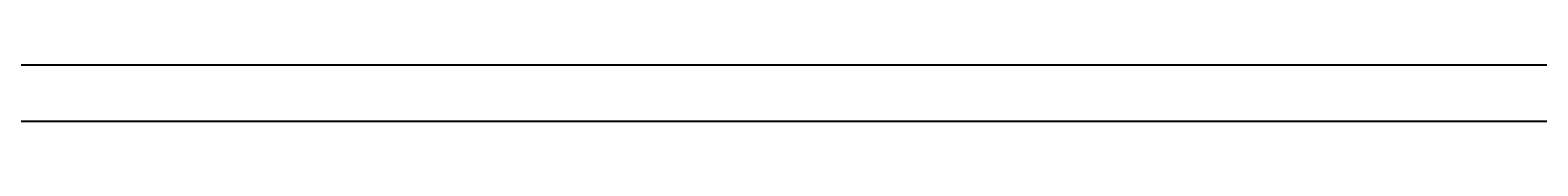
# Model space of a CAD drawing. Units: inches. Extents: x 35362 to 73946, y 43607 to 67532.
# Tile 117 of 134: x 50761 to 50905, y 49313 to 49321. Entities that reach past the tile are written whole.
import ezdxf

# ---------------------------------------------------------------- set-up
doc = ezdxf.new("R2010")
doc.units = ezdxf.units.IN
doc.header["$MEASUREMENT"] = 0
doc.layers.add('A-ANNO-DIMS', color=2, linetype='Continuous', lineweight=18)
doc.styles.get("Standard").update_dxf_attribs({"font": 'arial.ttf'})
doc.dimstyles.get("Standard").update_dxf_attribs({"dimtxt": 0.18, "dimasz": 0.18, "dimexe": 0.18, "dimexo": 0.0625, "dimgap": 0.09, "dimtad": 0, "dimtih": 1, "dimtoh": 1, "dimdec": 4, "dimzin": 0, "dimdsep": 46, "dimtxsty": 'Standard', "dimcen": 0.09, "dimadec": 0, "dimazin": 0, "dimtfac": 1, "dimtdec": 4, "dimtofl": 0, "dimtmove": 0, "dimatfit": 3, "dimfxl": 1, "dimtolj": 1, "dimtzin": 0, "dimarcsym": 0})

# ---------------------------------------------------------------- blocks, each defined once
blk = doc.blocks.new('*D11')
at = {"layer": 'A-ANNO-DIMS', "color": 0, "lineweight": -2, "transparency": 16777216}
for p, q in [((47978.66, 56028.77), (47978.66, 43606.68)), ((53109.76, 56028.77), (53109.76, 43606.68)), ((47978.84, 43606.86), (50543.87, 43606.86)), ((53109.58, 43606.86), (50544.55, 43606.86))]:
    blk.add_line(p, q, dxfattribs=at)
at = {"layer": 'A-ANNO-DIMS', "color": 0, "transparency": 16777216}
for points in [[(47978.84, 43606.89), (47978.84, 43606.83), (47978.66, 43606.86)], [(53109.58, 43606.89), (53109.58, 43606.83), (53109.76, 43606.86)]]:
    blk.add_solid(points, dxfattribs=at)
at = {"layer": 'Defpoints', "color": 0, "transparency": 16777216}
for p in [(47978.66, 56028.84), (53109.76, 56028.84), (53109.76, 43606.86)]:
    blk.add_point(p, dxfattribs=at)
at = {"layer": 'A-ANNO-DIMS', "color": 0, "transparency": 16777216, "insert": (50544.21, 43606.86), "char_height": 0.18, "attachment_point": 5}
blk.add_mtext('\\A1;5131', dxfattribs=at)
blk = doc.blocks.new('*D13')
at = {"layer": 'A-ANNO-DIMS', "color": 0, "lineweight": -2, "transparency": 16777216}
for p, q in [((48373.49, 51694.02), (48373.49, 43606.68)), ((51029.04, 51694.02), (51029.04, 43606.68)), ((48373.67, 43606.86), (49700.8, 43606.86)), ((51028.86, 43606.86), (49701.73, 43606.86))]:
    blk.add_line(p, q, dxfattribs=at)
at = {"layer": 'A-ANNO-DIMS', "color": 0, "transparency": 16777216}
for points in [[(48373.67, 43606.89), (48373.67, 43606.83), (48373.49, 43606.86)], [(51028.86, 43606.89), (51028.86, 43606.83), (51029.04, 43606.86)]]:
    blk.add_solid(points, dxfattribs=at)
at = {"layer": 'Defpoints', "color": 0, "transparency": 16777216}
for p in [(48373.49, 51694.09), (51029.04, 51694.09), (51029.04, 43606.86)]:
    blk.add_point(p, dxfattribs=at)
at = {"layer": 'A-ANNO-DIMS', "color": 0, "transparency": 16777216, "insert": (49701.27, 43606.86), "char_height": 0.18, "attachment_point": 5}
blk.add_mtext('\\A1;2655.6', dxfattribs=at)
blk = doc.blocks.new('*D17')
at = {"layer": 'A-ANNO-DIMS', "color": 0, "lineweight": -2, "transparency": 16777216}
for p, q in [((49923.31, 61293.22), (49923.31, 43606.68)), ((51913.93, 61293.22), (51913.93, 43606.68)), ((49923.49, 43606.86), (50918.16, 43606.86)), ((51913.75, 43606.86), (50919.07, 43606.86))]:
    blk.add_line(p, q, dxfattribs=at)
at = {"layer": 'A-ANNO-DIMS', "color": 0, "transparency": 16777216}
for points in [[(49923.49, 43606.89), (49923.49, 43606.83), (49923.31, 43606.86)], [(51913.75, 43606.89), (51913.75, 43606.83), (51913.93, 43606.86)]]:
    blk.add_solid(points, dxfattribs=at)
at = {"layer": 'Defpoints', "color": 0, "transparency": 16777216}
for p in [(49923.31, 61293.29), (51913.93, 61293.29), (51913.93, 43606.86)]:
    blk.add_point(p, dxfattribs=at)
at = {"layer": 'A-ANNO-DIMS', "color": 0, "transparency": 16777216, "insert": (50918.62, 43606.86), "char_height": 0.18, "attachment_point": 5}
blk.add_mtext('\\A1;1990.6', dxfattribs=at)
blk = doc.blocks.new('*D40')
at = {"layer": 'A-ANNO-DIMS', "color": 0, "lineweight": -2, "transparency": 16777216}
for p, q in [((56873.54, 53351.53), (35361.77, 53351.53)), ((35361.95, 53351.35), (35361.95, 51333.28)), ((35361.95, 49314.85), (35361.95, 51332.92)), ((51806.45, 49314.67), (35361.77, 49314.67))]:
    blk.add_line(p, q, dxfattribs=at)
at = {"layer": 'A-ANNO-DIMS', "color": 0, "transparency": 16777216}
for points in [[(35361.92, 53351.35), (35361.98, 53351.35), (35361.95, 53351.53)], [(35361.92, 49314.85), (35361.98, 49314.85), (35361.95, 49314.67)]]:
    blk.add_solid(points, dxfattribs=at)
at = {"layer": 'Defpoints', "color": 0, "transparency": 16777216}
for p in [(35361.95, 53351.53), (56873.6, 53351.53), (51806.52, 49314.67)]:
    blk.add_point(p, dxfattribs=at)
at = {"layer": 'A-ANNO-DIMS', "color": 0, "transparency": 16777216, "insert": (35361.95, 51333.1), "char_height": 0.18, "attachment_point": 5}
blk.add_mtext('\\A1;4036.9', dxfattribs=at)
blk = doc.blocks.new('*D67')
at = {"layer": 'A-ANNO-DIMS', "color": 0, "lineweight": -2, "transparency": 16777216}
for p, q in [((56873.54, 53351.53), (35361.77, 53351.53)), ((35361.95, 53351.35), (35361.95, 49400.89)), ((35361.95, 45450.07), (35361.95, 49400.53)), ((53793.58, 45449.89), (35361.77, 45449.89))]:
    blk.add_line(p, q, dxfattribs=at)
at = {"layer": 'A-ANNO-DIMS', "color": 0, "transparency": 16777216}
for points in [[(35361.92, 53351.35), (35361.98, 53351.35), (35361.95, 53351.53)], [(35361.92, 45450.07), (35361.98, 45450.07), (35361.95, 45449.89)]]:
    blk.add_solid(points, dxfattribs=at)
at = {"layer": 'Defpoints', "color": 0, "transparency": 16777216}
for p in [(35361.95, 53351.53), (56873.6, 53351.53), (53793.64, 45449.89)]:
    blk.add_point(p, dxfattribs=at)
at = {"layer": 'A-ANNO-DIMS', "color": 0, "transparency": 16777216, "insert": (35361.95, 49400.71), "char_height": 0.18, "attachment_point": 5}
blk.add_mtext('\\A1;7901.6', dxfattribs=at)
blk = doc.blocks.new('*D86')
at = {"layer": 'A-ANNO-DIMS', "color": 0, "lineweight": -2, "transparency": 16777216}
for p, q in [((51285.53, 49320.08), (35361.77, 49320.08)), ((35361.95, 49319.9), (35361.95, 49120.26)), ((35361.95, 48920.26), (35361.95, 49119.9)), ((51285.53, 48920.08), (35361.77, 48920.08))]:
    blk.add_line(p, q, dxfattribs=at)
at = {"layer": 'A-ANNO-DIMS', "color": 0, "transparency": 16777216}
for points in [[(35361.92, 49319.9), (35361.98, 49319.9), (35361.95, 49320.08)], [(35361.92, 48920.26), (35361.98, 48920.26), (35361.95, 48920.08)]]:
    blk.add_solid(points, dxfattribs=at)
at = {"layer": 'Defpoints', "color": 0, "transparency": 16777216}
for p in [(35361.95, 49320.08), (51285.59, 49320.08), (51285.59, 48920.08)]:
    blk.add_point(p, dxfattribs=at)
at = {"layer": 'A-ANNO-DIMS', "color": 0, "transparency": 16777216, "insert": (35361.95, 49120.08), "char_height": 0.18, "attachment_point": 5}
blk.add_mtext('\\A1;400.0', dxfattribs=at)
blk = doc.blocks.new('*D107')
at = {"layer": 'A-ANNO-DIMS', "color": 0, "lineweight": -2, "transparency": 16777216}
for p, q in [((50139.56, 59850.01), (50139.56, 43606.68)), ((51320.81, 59850.01), (51320.81, 43606.68)), ((50139.74, 43606.86), (50729.73, 43606.86)), ((51320.63, 43606.86), (50730.64, 43606.86))]:
    blk.add_line(p, q, dxfattribs=at)
at = {"layer": 'A-ANNO-DIMS', "color": 0, "transparency": 16777216}
for points in [[(50139.74, 43606.89), (50139.74, 43606.83), (50139.56, 43606.86)], [(51320.63, 43606.89), (51320.63, 43606.83), (51320.81, 43606.86)]]:
    blk.add_solid(points, dxfattribs=at)
at = {"layer": 'Defpoints', "color": 0, "transparency": 16777216}
for p in [(50139.56, 59850.08), (51320.81, 59850.08), (51320.81, 43606.86)]:
    blk.add_point(p, dxfattribs=at)
at = {"layer": 'A-ANNO-DIMS', "color": 0, "transparency": 16777216, "insert": (50730.19, 43606.86), "char_height": 0.18, "attachment_point": 5}
blk.add_mtext('\\A1;1181.3', dxfattribs=at)

msp = doc.modelspace()

# ---------------------------------------------------------------- dimensions: what is measured, and where the dimension line sits
at = {"layer": 'A-ANNO-DIMS'}
for base, p1, p2, override, picture, middle in [((51913.931, 43606.859), (49923.307, 61293.286), (51913.931, 61293.286), {"dimdec": 1, "dimlfac": 1, "dimrnd": 0, "dimzin": 0, "dimdsep": 46, "dimlunit": 2}, '*D17', (50918.619, 43606.859)), ((51320.8133, 43606.859), (50139.5627, 59850.0769), (51320.8133, 59850.0769), {"dimdec": 1, "dimlfac": 1, "dimrnd": 0, "dimzin": 0, "dimdsep": 46, "dimlunit": 2}, '*D107', (50730.188, 43606.859)), ((53109.76, 43606.859), (47978.665, 56028.836), (53109.76, 56028.836), {"dimdec": 0, "dimlfac": 1, "dimrnd": 0, "dimzin": 0, "dimdsep": 46, "dimlunit": 2}, '*D11', (50544.212, 43606.859)), ((51029.043, 43606.859), (48373.492, 51694.087), (51029.043, 51694.087), {"dimdec": 1, "dimlfac": 1, "dimrnd": 0, "dimzin": 0, "dimdsep": 46, "dimlunit": 2}, '*D13', (49701.267, 43606.859))]:
    dim = msp.add_linear_dim(base=base, p1=p1, p2=p2, dimstyle='Standard', override=override, dxfattribs=at)
    dim.commit()
    dim.dimension.update_dxf_attribs({"geometry": picture, "text_midpoint": middle})
for base, p1, p2, picture, middle in [((35361.949, 53351.529), (51806.517, 49314.669), (56873.602, 53351.529), '*D40', (35361.949, 51333.099)), ((35361.949, 53351.529), (53793.638, 45449.894), (56873.602, 53351.529), '*D67', (35361.949, 49400.712)), ((35361.949, 49320.079), (51285.595, 48920.079), (51285.595, 49320.079), '*D86', (35361.949, 49120.079))]:
    dim = msp.add_linear_dim(base=base, p1=p1, p2=p2, angle=90, dimstyle='Standard', override={"dimdec": 1, "dimlfac": 1, "dimrnd": 0, "dimzin": 0, "dimdsep": 46, "dimlunit": 2}, dxfattribs=at)
    dim.commit()
    dim.dimension.update_dxf_attribs({"geometry": picture, "text_midpoint": middle})

doc.saveas('drawing.dxf')
